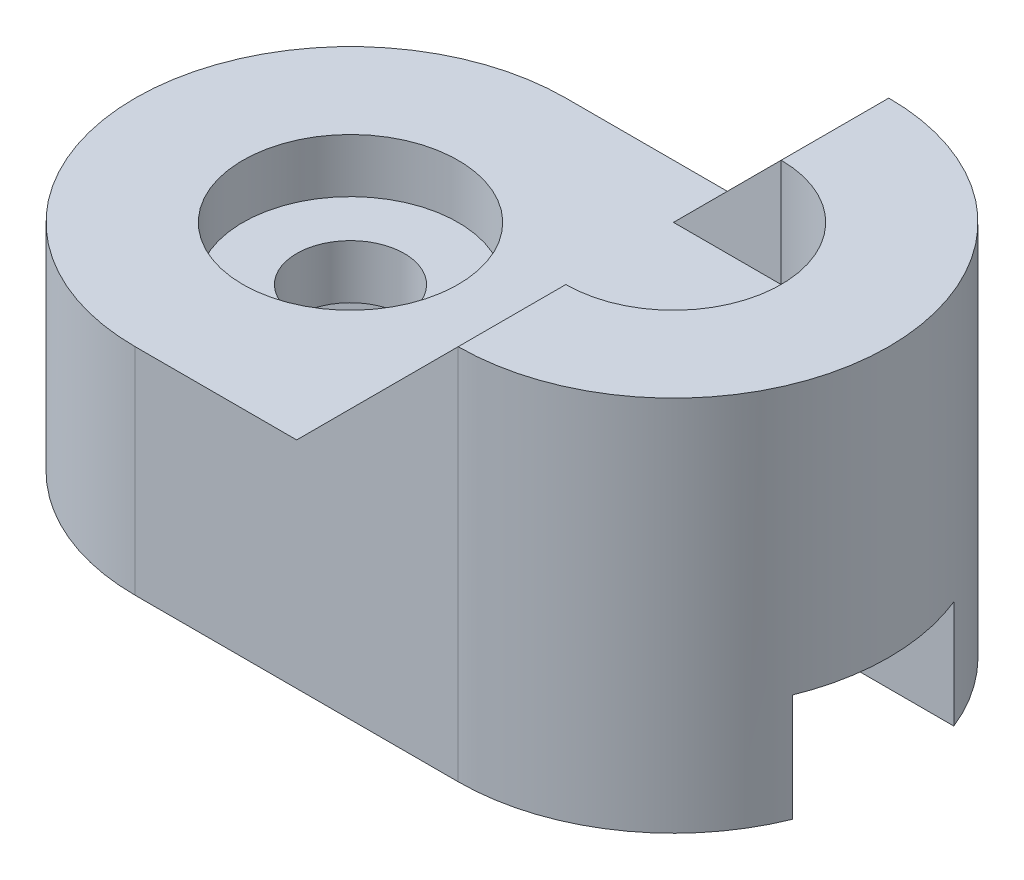
ISO-10303-21;
HEADER;
FILE_DESCRIPTION(('STEP AP214'),'2;1');
FILE_NAME('part.step','',(''),(''),'','','');
FILE_SCHEMA(('AUTOMOTIVE_DESIGN { 1 0 10303 214 1 1 1 1 }'));
ENDSEC;
DATA;
#1=APPLICATION_CONTEXT('core data for automotive mechanical design processes');
#2=APPLICATION_PROTOCOL_DEFINITION('international standard','automotive_design',2000,#1);
#3=PRODUCT_CONTEXT('',#1,'mechanical');
#4=PRODUCT('Part','Part','',(#3));
#5=PRODUCT_RELATED_PRODUCT_CATEGORY('part','',(#4));
#6=PRODUCT_DEFINITION_FORMATION('','',#4);
#7=PRODUCT_DEFINITION_CONTEXT('part definition',#1,'design');
#8=PRODUCT_DEFINITION('design','',#6,#7);
#9=PRODUCT_DEFINITION_SHAPE('','',#8);
#10=(LENGTH_UNIT() NAMED_UNIT(*) SI_UNIT(.MILLI.,.METRE.));
#11=(NAMED_UNIT(*) PLANE_ANGLE_UNIT() SI_UNIT($,.RADIAN.));
#12=(NAMED_UNIT(*) SI_UNIT($,.STERADIAN.) SOLID_ANGLE_UNIT());
#13=UNCERTAINTY_MEASURE_WITH_UNIT(LENGTH_MEASURE(1.E-05),#10,'distance_accuracy_value','');
#14=(GEOMETRIC_REPRESENTATION_CONTEXT(3) GLOBAL_UNCERTAINTY_ASSIGNED_CONTEXT((#13)) GLOBAL_UNIT_ASSIGNED_CONTEXT((#10,
#11,#12)) REPRESENTATION_CONTEXT('',''));
#15=CARTESIAN_POINT('',(0.,0.,0.));
#16=DIRECTION('',(0.,0.,1.));
#17=DIRECTION('',(1.,0.,0.));
#18=AXIS2_PLACEMENT_3D('',#15,#16,#17);
#19=CARTESIAN_POINT('',(0.,70.,-40.));
#20=DIRECTION('',(1.,0.,0.));
#21=DIRECTION('',(0.,0.,-1.));
#22=AXIS2_PLACEMENT_3D('',#19,#20,#21);
#23=PLANE('',#22);
#24=DIRECTION('',(0.,0.,1.));
#25=VECTOR('',#24,1.);
#26=CARTESIAN_POINT('',(0.,40.,-40.));
#27=LINE('',#26,#25);
#28=CARTESIAN_POINT('',(0.,40.,-30.));
#29=VERTEX_POINT('',#28);
#30=CARTESIAN_POINT('',(0.,40.,-20.));
#31=VERTEX_POINT('',#30);
#32=EDGE_CURVE('E167',#29,#31,#27,.T.);
#33=ORIENTED_EDGE('',*,*,#32,.T.);
#34=DIRECTION('',(0.,1.,0.));
#35=VECTOR('',#34,1.);
#36=CARTESIAN_POINT('',(0.,70.,-20.));
#37=LINE('',#36,#35);
#38=CARTESIAN_POINT('',(0.,70.,-20.));
#39=VERTEX_POINT('',#38);
#40=EDGE_CURVE('E52',#31,#39,#37,.T.);
#41=ORIENTED_EDGE('',*,*,#40,.T.);
#42=DIRECTION('',(0.,0.,1.));
#43=VECTOR('',#42,1.);
#44=CARTESIAN_POINT('',(0.,70.,-40.));
#45=LINE('',#44,#43);
#46=CARTESIAN_POINT('',(0.,70.,-30.));
#47=VERTEX_POINT('',#46);
#48=EDGE_CURVE('E154',#47,#39,#45,.T.);
#49=ORIENTED_EDGE('',*,*,#48,.F.);
#50=DIRECTION('',(0.,1.,0.));
#51=VECTOR('',#50,1.);
#52=CARTESIAN_POINT('',(0.,70.,-30.));
#53=LINE('',#52,#51);
#54=EDGE_CURVE('E236',#29,#47,#53,.T.);
#55=ORIENTED_EDGE('',*,*,#54,.F.);
#56=EDGE_LOOP('',(#33,#41,#49,#55));
#57=FACE_BOUND('',#56,.T.);
#58=ADVANCED_FACE('F39',(#57),#23,.F.);
#59=CARTESIAN_POINT('',(0.,70.,0.));
#60=DIRECTION('',(0.,-1.,0.));
#61=DIRECTION('',(0.,0.,-1.));
#62=AXIS2_PLACEMENT_3D('',#59,#60,#61);
#63=PLANE('',#62);
#64=CARTESIAN_POINT('',(0.,70.,0.));
#65=DIRECTION('',(0.,1.,0.));
#66=DIRECTION('',(0.,0.,1.));
#67=AXIS2_PLACEMENT_3D('',#64,#65,#66);
#68=CIRCLE('',#67,20.);
#69=CARTESIAN_POINT('',(0.,70.,20.));
#70=VERTEX_POINT('',#69);
#71=EDGE_CURVE('E143',#70,#39,#68,.T.);
#72=ORIENTED_EDGE('',*,*,#71,.F.);
#73=CARTESIAN_POINT('',(0.,70.,30.));
#74=VERTEX_POINT('',#73);
#75=EDGE_CURVE('E151',#70,#74,#45,.T.);
#76=ORIENTED_EDGE('',*,*,#75,.T.);
#77=DIRECTION('',(0.,0.,1.));
#78=VECTOR('',#77,1.);
#79=CARTESIAN_POINT('',(0.,70.,40.));
#80=LINE('',#79,#78);
#81=CARTESIAN_POINT('',(0.,70.,40.));
#82=VERTEX_POINT('',#81);
#83=EDGE_CURVE('E249',#74,#82,#80,.T.);
#84=ORIENTED_EDGE('',*,*,#83,.T.);
#85=CARTESIAN_POINT('',(0.,70.,0.));
#86=DIRECTION('',(0.,1.,0.));
#87=DIRECTION('',(0.,0.,-1.));
#88=AXIS2_PLACEMENT_3D('',#85,#86,#87);
#89=CIRCLE('',#88,40.);
#90=CARTESIAN_POINT('',(0.,70.,-40.));
#91=VERTEX_POINT('',#90);
#92=EDGE_CURVE('E165',#82,#91,#89,.T.);
#93=ORIENTED_EDGE('',*,*,#92,.T.);
#94=EDGE_CURVE('E163',#91,#47,#45,.T.);
#95=ORIENTED_EDGE('',*,*,#94,.T.);
#96=ORIENTED_EDGE('',*,*,#48,.T.);
#97=EDGE_LOOP('',(#72,#76,#84,#93,#95,#96));
#98=FACE_BOUND('',#97,.T.);
#99=ADVANCED_FACE('F149',(#98),#63,.F.);
#100=ORIENTED_EDGE('',*,*,#75,.F.);
#101=DIRECTION('',(0.,1.,0.));
#102=VECTOR('',#101,1.);
#103=CARTESIAN_POINT('',(0.,70.,20.));
#104=LINE('',#103,#102);
#105=CARTESIAN_POINT('',(0.,40.,20.));
#106=VERTEX_POINT('',#105);
#107=EDGE_CURVE('E140',#70,#106,#104,.F.);
#108=ORIENTED_EDGE('',*,*,#107,.T.);
#109=CARTESIAN_POINT('',(0.,40.,30.));
#110=VERTEX_POINT('',#109);
#111=EDGE_CURVE('E272',#106,#110,#27,.T.);
#112=ORIENTED_EDGE('',*,*,#111,.T.);
#113=DIRECTION('',(0.,-1.,0.));
#114=VECTOR('',#113,1.);
#115=CARTESIAN_POINT('',(0.,70.,30.));
#116=LINE('',#115,#114);
#117=EDGE_CURVE('E161',#74,#110,#116,.T.);
#118=ORIENTED_EDGE('',*,*,#117,.F.);
#119=EDGE_LOOP('',(#100,#108,#112,#118));
#120=FACE_BOUND('',#119,.T.);
#121=ADVANCED_FACE('F157',(#120),#23,.F.);
#122=CARTESIAN_POINT('',(0.,0.,0.));
#123=DIRECTION('',(0.,1.,0.));
#124=DIRECTION('',(0.,0.,1.));
#125=AXIS2_PLACEMENT_3D('',#122,#123,#124);
#126=PLANE('',#125);
#127=DIRECTION('',(1.,0.,0.));
#128=VECTOR('',#127,1.);
#129=CARTESIAN_POINT('',(0.,0.,40.));
#130=LINE('',#129,#128);
#131=CARTESIAN_POINT('',(-60.,0.,40.));
#132=VERTEX_POINT('',#131);
#133=CARTESIAN_POINT('',(0.,0.,40.));
#134=VERTEX_POINT('',#133);
#135=EDGE_CURVE('E187',#132,#134,#130,.T.);
#136=ORIENTED_EDGE('',*,*,#135,.F.);
#137=CARTESIAN_POINT('',(-60.,0.,0.));
#138=DIRECTION('',(0.,1.,0.));
#139=DIRECTION('',(0.,0.,1.));
#140=AXIS2_PLACEMENT_3D('',#137,#138,#139);
#141=CIRCLE('',#140,40.);
#142=CARTESIAN_POINT('',(-97.0809924354783,0.,15.));
#143=VERTEX_POINT('',#142);
#144=EDGE_CURVE('E181',#143,#132,#141,.T.);
#145=ORIENTED_EDGE('',*,*,#144,.F.);
#146=DIRECTION('',(1.,0.,0.));
#147=VECTOR('',#146,1.);
#148=CARTESIAN_POINT('',(0.,0.,15.));
#149=LINE('',#148,#147);
#150=CARTESIAN_POINT('',(37.0809924354783,0.,15.));
#151=VERTEX_POINT('',#150);
#152=EDGE_CURVE('E201',#143,#151,#149,.T.);
#153=ORIENTED_EDGE('',*,*,#152,.T.);
#154=CARTESIAN_POINT('',(0.,0.,0.));
#155=DIRECTION('',(0.,1.,0.));
#156=DIRECTION('',(0.,0.,1.));
#157=AXIS2_PLACEMENT_3D('',#154,#155,#156);
#158=CIRCLE('',#157,40.);
#159=EDGE_CURVE('E168',#134,#151,#158,.T.);
#160=ORIENTED_EDGE('',*,*,#159,.F.);
#161=EDGE_LOOP('',(#136,#145,#153,#160));
#162=FACE_BOUND('',#161,.T.);
#163=ADVANCED_FACE('F327',(#162),#126,.F.);
#164=CARTESIAN_POINT('',(0.,40.,0.));
#165=DIRECTION('',(0.,-1.,0.));
#166=DIRECTION('',(0.,0.,-1.));
#167=AXIS2_PLACEMENT_3D('',#164,#165,#166);
#168=CYLINDRICAL_SURFACE('',#167,40.);
#169=DIRECTION('',(0.,-1.,0.));
#170=VECTOR('',#169,1.);
#171=CARTESIAN_POINT('',(0.,40.,-40.));
#172=LINE('',#171,#170);
#173=CARTESIAN_POINT('',(0.,0.,-40.));
#174=VERTEX_POINT('',#173);
#175=EDGE_CURVE('E197',#91,#174,#172,.T.);
#176=ORIENTED_EDGE('',*,*,#175,.F.);
#177=ORIENTED_EDGE('',*,*,#92,.F.);
#178=DIRECTION('',(0.,-1.,0.));
#179=VECTOR('',#178,1.);
#180=CARTESIAN_POINT('',(0.,40.,40.));
#181=LINE('',#180,#179);
#182=EDGE_CURVE('E186',#82,#134,#181,.T.);
#183=ORIENTED_EDGE('',*,*,#182,.T.);
#184=ORIENTED_EDGE('',*,*,#159,.T.);
#185=DIRECTION('',(0.,-1.,0.));
#186=VECTOR('',#185,1.);
#187=CARTESIAN_POINT('',(37.0809924354783,40.,15.));
#188=LINE('',#187,#186);
#189=CARTESIAN_POINT('',(37.0809924354783,20.,15.));
#190=VERTEX_POINT('',#189);
#191=EDGE_CURVE('E267',#151,#190,#188,.F.);
#192=ORIENTED_EDGE('',*,*,#191,.T.);
#193=CARTESIAN_POINT('',(0.,20.,0.));
#194=DIRECTION('',(0.,1.,0.));
#195=DIRECTION('',(0.,0.,1.));
#196=AXIS2_PLACEMENT_3D('',#193,#194,#195);
#197=CIRCLE('',#196,40.);
#198=CARTESIAN_POINT('',(37.0809924354783,20.,-15.));
#199=VERTEX_POINT('',#198);
#200=EDGE_CURVE('E275',#190,#199,#197,.T.);
#201=ORIENTED_EDGE('',*,*,#200,.T.);
#202=DIRECTION('',(0.,-1.,0.));
#203=VECTOR('',#202,1.);
#204=CARTESIAN_POINT('',(37.0809924354783,40.,-15.));
#205=LINE('',#204,#203);
#206=CARTESIAN_POINT('',(37.0809924354783,0.,-15.));
#207=VERTEX_POINT('',#206);
#208=EDGE_CURVE('E262',#199,#207,#205,.T.);
#209=ORIENTED_EDGE('',*,*,#208,.T.);
#210=EDGE_CURVE('E166',#207,#174,#158,.T.);
#211=ORIENTED_EDGE('',*,*,#210,.T.);
#212=EDGE_LOOP('',(#176,#177,#183,#184,#192,#201,#209,#211));
#213=FACE_BOUND('',#212,.T.);
#214=ADVANCED_FACE('F41',(#213),#168,.T.);
#215=CARTESIAN_POINT('',(0.,40.,-40.));
#216=DIRECTION('',(0.,0.,1.));
#217=DIRECTION('',(1.,0.,0.));
#218=AXIS2_PLACEMENT_3D('',#215,#216,#217);
#219=PLANE('',#218);
#220=DIRECTION('',(-1.,0.,0.));
#221=VECTOR('',#220,1.);
#222=CARTESIAN_POINT('',(0.,0.,-40.));
#223=LINE('',#222,#221);
#224=CARTESIAN_POINT('',(-60.,0.,-40.));
#225=VERTEX_POINT('',#224);
#226=EDGE_CURVE('E179',#174,#225,#223,.T.);
#227=ORIENTED_EDGE('',*,*,#226,.T.);
#228=DIRECTION('',(0.,-1.,0.));
#229=VECTOR('',#228,1.);
#230=CARTESIAN_POINT('',(-60.,40.,-40.));
#231=LINE('',#230,#229);
#232=CARTESIAN_POINT('',(-60.,40.,-40.));
#233=VERTEX_POINT('',#232);
#234=EDGE_CURVE('E192',#233,#225,#231,.T.);
#235=ORIENTED_EDGE('',*,*,#234,.F.);
#236=DIRECTION('',(-1.,0.,0.));
#237=VECTOR('',#236,1.);
#238=CARTESIAN_POINT('',(0.,40.,-40.));
#239=LINE('',#238,#237);
#240=CARTESIAN_POINT('',(-30.,40.,-40.));
#241=VERTEX_POINT('',#240);
#242=EDGE_CURVE('E190',#241,#233,#239,.T.);
#243=ORIENTED_EDGE('',*,*,#242,.F.);
#244=DIRECTION('',(0.707106781186547,0.707106781186548,0.));
#245=VECTOR('',#244,1.);
#246=CARTESIAN_POINT('',(0.,70.,-40.));
#247=LINE('',#246,#245);
#248=EDGE_CURVE('E234',#241,#91,#247,.T.);
#249=ORIENTED_EDGE('',*,*,#248,.T.);
#250=ORIENTED_EDGE('',*,*,#175,.T.);
#251=EDGE_LOOP('',(#227,#235,#243,#249,#250));
#252=FACE_BOUND('',#251,.T.);
#253=ADVANCED_FACE('F299',(#252),#219,.F.);
#254=CARTESIAN_POINT('',(-60.,40.,0.));
#255=DIRECTION('',(0.,-1.,0.));
#256=DIRECTION('',(0.,0.,-1.));
#257=AXIS2_PLACEMENT_3D('',#254,#255,#256);
#258=CYLINDRICAL_SURFACE('',#257,40.);
#259=ORIENTED_EDGE('',*,*,#234,.T.);
#260=CARTESIAN_POINT('',(-97.0809924354783,0.,-15.));
#261=VERTEX_POINT('',#260);
#262=EDGE_CURVE('E184',#225,#261,#141,.T.);
#263=ORIENTED_EDGE('',*,*,#262,.T.);
#264=DIRECTION('',(0.,-1.,0.));
#265=VECTOR('',#264,1.);
#266=CARTESIAN_POINT('',(-97.0809924354783,40.,-15.));
#267=LINE('',#266,#265);
#268=CARTESIAN_POINT('',(-97.0809924354783,20.,-15.));
#269=VERTEX_POINT('',#268);
#270=EDGE_CURVE('E259',#261,#269,#267,.F.);
#271=ORIENTED_EDGE('',*,*,#270,.T.);
#272=CARTESIAN_POINT('',(-60.,20.,0.));
#273=DIRECTION('',(0.,1.,0.));
#274=DIRECTION('',(0.,0.,1.));
#275=AXIS2_PLACEMENT_3D('',#272,#273,#274);
#276=CIRCLE('',#275,40.);
#277=CARTESIAN_POINT('',(-97.0809924354783,20.,15.));
#278=VERTEX_POINT('',#277);
#279=EDGE_CURVE('E50',#269,#278,#276,.T.);
#280=ORIENTED_EDGE('',*,*,#279,.T.);
#281=DIRECTION('',(0.,-1.,0.));
#282=VECTOR('',#281,1.);
#283=CARTESIAN_POINT('',(-97.0809924354783,40.,15.));
#284=LINE('',#283,#282);
#285=EDGE_CURVE('E266',#278,#143,#284,.T.);
#286=ORIENTED_EDGE('',*,*,#285,.T.);
#287=ORIENTED_EDGE('',*,*,#144,.T.);
#288=DIRECTION('',(0.,-1.,0.));
#289=VECTOR('',#288,1.);
#290=CARTESIAN_POINT('',(-60.,40.,40.));
#291=LINE('',#290,#289);
#292=CARTESIAN_POINT('',(-60.,40.,40.));
#293=VERTEX_POINT('',#292);
#294=EDGE_CURVE('E191',#293,#132,#291,.T.);
#295=ORIENTED_EDGE('',*,*,#294,.F.);
#296=CARTESIAN_POINT('',(-60.,40.,0.));
#297=DIRECTION('',(0.,1.,0.));
#298=DIRECTION('',(0.,0.,1.));
#299=AXIS2_PLACEMENT_3D('',#296,#297,#298);
#300=CIRCLE('',#299,40.);
#301=EDGE_CURVE('E280',#233,#293,#300,.T.);
#302=ORIENTED_EDGE('',*,*,#301,.F.);
#303=EDGE_LOOP('',(#259,#263,#271,#280,#286,#287,#295,#302));
#304=FACE_BOUND('',#303,.T.);
#305=ADVANCED_FACE('F359',(#304),#258,.T.);
#306=CARTESIAN_POINT('',(0.,40.,40.));
#307=DIRECTION('',(0.,0.,-1.));
#308=DIRECTION('',(-1.,0.,0.));
#309=AXIS2_PLACEMENT_3D('',#306,#307,#308);
#310=PLANE('',#309);
#311=ORIENTED_EDGE('',*,*,#294,.T.);
#312=ORIENTED_EDGE('',*,*,#135,.T.);
#313=ORIENTED_EDGE('',*,*,#182,.F.);
#314=DIRECTION('',(0.707106781186547,0.707106781186548,0.));
#315=VECTOR('',#314,1.);
#316=CARTESIAN_POINT('',(0.,70.,40.));
#317=LINE('',#316,#315);
#318=CARTESIAN_POINT('',(-30.,40.,40.));
#319=VERTEX_POINT('',#318);
#320=EDGE_CURVE('E245',#319,#82,#317,.T.);
#321=ORIENTED_EDGE('',*,*,#320,.F.);
#322=DIRECTION('',(1.,0.,0.));
#323=VECTOR('',#322,1.);
#324=CARTESIAN_POINT('',(0.,40.,40.));
#325=LINE('',#324,#323);
#326=EDGE_CURVE('E178',#293,#319,#325,.T.);
#327=ORIENTED_EDGE('',*,*,#326,.F.);
#328=EDGE_LOOP('',(#311,#312,#313,#321,#327));
#329=FACE_BOUND('',#328,.T.);
#330=ADVANCED_FACE('F290',(#329),#310,.F.);
#331=CARTESIAN_POINT('',(0.,40.,0.));
#332=DIRECTION('',(0.,1.,0.));
#333=DIRECTION('',(0.,0.,1.));
#334=AXIS2_PLACEMENT_3D('',#331,#332,#333);
#335=PLANE('',#334);
#336=CARTESIAN_POINT('',(0.,40.,0.));
#337=DIRECTION('',(0.,1.,0.));
#338=DIRECTION('',(0.,0.,1.));
#339=AXIS2_PLACEMENT_3D('',#336,#337,#338);
#340=CIRCLE('',#339,20.);
#341=EDGE_CURVE('E11',#31,#106,#340,.T.);
#342=ORIENTED_EDGE('',*,*,#341,.F.);
#343=ORIENTED_EDGE('',*,*,#32,.F.);
#344=DIRECTION('',(-1.,0.,0.));
#345=VECTOR('',#344,1.);
#346=CARTESIAN_POINT('',(0.,40.,-30.));
#347=LINE('',#346,#345);
#348=CARTESIAN_POINT('',(-30.,40.,-30.));
#349=VERTEX_POINT('',#348);
#350=EDGE_CURVE('E233',#29,#349,#347,.T.);
#351=ORIENTED_EDGE('',*,*,#350,.T.);
#352=DIRECTION('',(0.,0.,1.));
#353=VECTOR('',#352,1.);
#354=CARTESIAN_POINT('',(-30.,40.,0.));
#355=LINE('',#354,#353);
#356=EDGE_CURVE('E238',#241,#349,#355,.T.);
#357=ORIENTED_EDGE('',*,*,#356,.F.);
#358=ORIENTED_EDGE('',*,*,#242,.T.);
#359=ORIENTED_EDGE('',*,*,#301,.T.);
#360=ORIENTED_EDGE('',*,*,#326,.T.);
#361=DIRECTION('',(0.,0.,-1.));
#362=VECTOR('',#361,1.);
#363=CARTESIAN_POINT('',(-30.,40.,0.));
#364=LINE('',#363,#362);
#365=CARTESIAN_POINT('',(-30.,40.,30.));
#366=VERTEX_POINT('',#365);
#367=EDGE_CURVE('E251',#366,#319,#364,.F.);
#368=ORIENTED_EDGE('',*,*,#367,.F.);
#369=DIRECTION('',(1.,0.,0.));
#370=VECTOR('',#369,1.);
#371=CARTESIAN_POINT('',(0.,40.,30.));
#372=LINE('',#371,#370);
#373=EDGE_CURVE('E247',#366,#110,#372,.T.);
#374=ORIENTED_EDGE('',*,*,#373,.T.);
#375=ORIENTED_EDGE('',*,*,#111,.F.);
#376=EDGE_LOOP('',(#342,#343,#351,#357,#358,#359,#360,#368,#374,#375));
#377=FACE_BOUND('',#376,.T.);
#378=CARTESIAN_POINT('',(-60.,40.,0.));
#379=DIRECTION('',(0.,1.,0.));
#380=DIRECTION('',(0.,0.,1.));
#381=AXIS2_PLACEMENT_3D('',#378,#379,#380);
#382=CIRCLE('',#381,20.);
#383=CARTESIAN_POINT('',(-60.,40.,20.));
#384=VERTEX_POINT('',#383);
#385=EDGE_CURVE('E224',#384,#384,#382,.T.);
#386=ORIENTED_EDGE('',*,*,#385,.F.);
#387=EDGE_LOOP('',(#386));
#388=FACE_BOUND('',#387,.T.);
#389=ADVANCED_FACE('F281',(#377,#388),#335,.T.);
#390=DIRECTION('',(-1.,0.,0.));
#391=VECTOR('',#390,1.);
#392=CARTESIAN_POINT('',(0.,0.,-15.));
#393=LINE('',#392,#391);
#394=EDGE_CURVE('E199',#207,#261,#393,.T.);
#395=ORIENTED_EDGE('',*,*,#394,.T.);
#396=ORIENTED_EDGE('',*,*,#262,.F.);
#397=ORIENTED_EDGE('',*,*,#226,.F.);
#398=ORIENTED_EDGE('',*,*,#210,.F.);
#399=EDGE_LOOP('',(#395,#396,#397,#398));
#400=FACE_BOUND('',#399,.T.);
#401=ADVANCED_FACE('F333',(#400),#126,.F.);
#402=CARTESIAN_POINT('',(-100.,20.,15.));
#403=DIRECTION('',(0.,1.,0.));
#404=DIRECTION('',(0.,0.,1.));
#405=AXIS2_PLACEMENT_3D('',#402,#403,#404);
#406=PLANE('',#405);
#407=CARTESIAN_POINT('',(0.,20.,0.));
#408=DIRECTION('',(0.,1.,0.));
#409=DIRECTION('',(0.,0.,1.));
#410=AXIS2_PLACEMENT_3D('',#407,#408,#409);
#411=CIRCLE('',#410,10.);
#412=CARTESIAN_POINT('',(0.,20.,10.));
#413=VERTEX_POINT('',#412);
#414=EDGE_CURVE('E144',#413,#413,#411,.T.);
#415=ORIENTED_EDGE('',*,*,#414,.T.);
#416=EDGE_LOOP('',(#415));
#417=FACE_BOUND('',#416,.T.);
#418=CARTESIAN_POINT('',(-60.,20.,0.));
#419=DIRECTION('',(0.,1.,0.));
#420=DIRECTION('',(0.,0.,1.));
#421=AXIS2_PLACEMENT_3D('',#418,#419,#420);
#422=CIRCLE('',#421,10.);
#423=CARTESIAN_POINT('',(-60.,20.,10.));
#424=VERTEX_POINT('',#423);
#425=EDGE_CURVE('E208',#424,#424,#422,.T.);
#426=ORIENTED_EDGE('',*,*,#425,.T.);
#427=EDGE_LOOP('',(#426));
#428=FACE_BOUND('',#427,.T.);
#429=DIRECTION('',(1.,0.,0.));
#430=VECTOR('',#429,1.);
#431=CARTESIAN_POINT('',(-100.,20.,15.));
#432=LINE('',#431,#430);
#433=EDGE_CURVE('E258',#278,#190,#432,.T.);
#434=ORIENTED_EDGE('',*,*,#433,.F.);
#435=ORIENTED_EDGE('',*,*,#279,.F.);
#436=DIRECTION('',(1.,0.,0.));
#437=VECTOR('',#436,1.);
#438=CARTESIAN_POINT('',(-100.,20.,-15.));
#439=LINE('',#438,#437);
#440=EDGE_CURVE('E254',#269,#199,#439,.T.);
#441=ORIENTED_EDGE('',*,*,#440,.T.);
#442=ORIENTED_EDGE('',*,*,#200,.F.);
#443=EDGE_LOOP('',(#434,#435,#441,#442));
#444=FACE_BOUND('',#443,.T.);
#445=ADVANCED_FACE('F345',(#417,#428,#444),#406,.F.);
#446=CARTESIAN_POINT('',(-100.,0.,15.));
#447=DIRECTION('',(0.,0.,1.));
#448=DIRECTION('',(1.,0.,0.));
#449=AXIS2_PLACEMENT_3D('',#446,#447,#448);
#450=PLANE('',#449);
#451=ORIENTED_EDGE('',*,*,#152,.F.);
#452=ORIENTED_EDGE('',*,*,#285,.F.);
#453=ORIENTED_EDGE('',*,*,#433,.T.);
#454=ORIENTED_EDGE('',*,*,#191,.F.);
#455=EDGE_LOOP('',(#451,#452,#453,#454));
#456=FACE_BOUND('',#455,.T.);
#457=ADVANCED_FACE('F349',(#456),#450,.F.);
#458=CARTESIAN_POINT('',(-100.,0.,-15.));
#459=DIRECTION('',(0.,0.,-1.));
#460=DIRECTION('',(-1.,0.,0.));
#461=AXIS2_PLACEMENT_3D('',#458,#459,#460);
#462=PLANE('',#461);
#463=ORIENTED_EDGE('',*,*,#440,.F.);
#464=ORIENTED_EDGE('',*,*,#270,.F.);
#465=ORIENTED_EDGE('',*,*,#394,.F.);
#466=ORIENTED_EDGE('',*,*,#208,.F.);
#467=EDGE_LOOP('',(#463,#464,#465,#466));
#468=FACE_BOUND('',#467,.T.);
#469=ADVANCED_FACE('F351',(#468),#462,.F.);
#470=CARTESIAN_POINT('',(0.,70.,40.));
#471=DIRECTION('',(0.707106781186548,-0.707106781186547,0.));
#472=DIRECTION('',(0.707106781186547,0.707106781186548,0.));
#473=AXIS2_PLACEMENT_3D('',#470,#471,#472);
#474=PLANE('',#473);
#475=DIRECTION('',(0.707106781186547,0.707106781186548,0.));
#476=VECTOR('',#475,1.);
#477=CARTESIAN_POINT('',(0.,70.,30.));
#478=LINE('',#477,#476);
#479=EDGE_CURVE('E244',#366,#74,#478,.T.);
#480=ORIENTED_EDGE('',*,*,#479,.F.);
#481=ORIENTED_EDGE('',*,*,#367,.T.);
#482=ORIENTED_EDGE('',*,*,#320,.T.);
#483=ORIENTED_EDGE('',*,*,#83,.F.);
#484=EDGE_LOOP('',(#480,#481,#482,#483));
#485=FACE_BOUND('',#484,.T.);
#486=ADVANCED_FACE('F291',(#485),#474,.F.);
#487=CARTESIAN_POINT('',(-30.,35.,30.));
#488=DIRECTION('',(0.,0.,1.));
#489=DIRECTION('',(1.,0.,0.));
#490=AXIS2_PLACEMENT_3D('',#487,#488,#489);
#491=PLANE('',#490);
#492=ORIENTED_EDGE('',*,*,#373,.F.);
#493=ORIENTED_EDGE('',*,*,#479,.T.);
#494=ORIENTED_EDGE('',*,*,#117,.T.);
#495=EDGE_LOOP('',(#492,#493,#494));
#496=FACE_BOUND('',#495,.T.);
#497=ADVANCED_FACE('F314',(#496),#491,.F.);
#498=CARTESIAN_POINT('',(-30.,35.,-30.));
#499=DIRECTION('',(0.,0.,-1.));
#500=DIRECTION('',(-1.,0.,0.));
#501=AXIS2_PLACEMENT_3D('',#498,#499,#500);
#502=PLANE('',#501);
#503=ORIENTED_EDGE('',*,*,#350,.F.);
#504=ORIENTED_EDGE('',*,*,#54,.T.);
#505=DIRECTION('',(0.707106781186547,0.707106781186548,0.));
#506=VECTOR('',#505,1.);
#507=CARTESIAN_POINT('',(0.,70.,-30.));
#508=LINE('',#507,#506);
#509=EDGE_CURVE('E62',#349,#47,#508,.T.);
#510=ORIENTED_EDGE('',*,*,#509,.F.);
#511=EDGE_LOOP('',(#503,#504,#510));
#512=FACE_BOUND('',#511,.T.);
#513=ADVANCED_FACE('F302',(#512),#502,.F.);
#514=CARTESIAN_POINT('',(0.,70.,-40.));
#515=DIRECTION('',(-0.707106781186548,0.707106781186547,0.));
#516=DIRECTION('',(0.707106781186547,0.707106781186548,0.));
#517=AXIS2_PLACEMENT_3D('',#514,#515,#516);
#518=PLANE('',#517);
#519=ORIENTED_EDGE('',*,*,#248,.F.);
#520=ORIENTED_EDGE('',*,*,#356,.T.);
#521=ORIENTED_EDGE('',*,*,#509,.T.);
#522=ORIENTED_EDGE('',*,*,#94,.F.);
#523=EDGE_LOOP('',(#519,#520,#521,#522));
#524=FACE_BOUND('',#523,.T.);
#525=ADVANCED_FACE('F301',(#524),#518,.T.);
#526=CARTESIAN_POINT('',(-60.,40.,0.));
#527=DIRECTION('',(0.,1.,0.));
#528=DIRECTION('',(0.,0.,1.));
#529=AXIS2_PLACEMENT_3D('',#526,#527,#528);
#530=CYLINDRICAL_SURFACE('',#529,10.);
#531=CARTESIAN_POINT('',(-60.,30.,0.));
#532=DIRECTION('',(0.,1.,0.));
#533=DIRECTION('',(0.,0.,1.));
#534=AXIS2_PLACEMENT_3D('',#531,#532,#533);
#535=CIRCLE('',#534,10.);
#536=CARTESIAN_POINT('',(-60.,30.,10.));
#537=VERTEX_POINT('',#536);
#538=EDGE_CURVE('E209',#537,#537,#535,.T.);
#539=ORIENTED_EDGE('',*,*,#538,.T.);
#540=EDGE_LOOP('',(#539));
#541=FACE_BOUND('',#540,.T.);
#542=ORIENTED_EDGE('',*,*,#425,.F.);
#543=EDGE_LOOP('',(#542));
#544=FACE_BOUND('',#543,.T.);
#545=ADVANCED_FACE('F303',(#541,#544),#530,.F.);
#546=CARTESIAN_POINT('',(-50.,30.,0.));
#547=DIRECTION('',(0.,-1.,0.));
#548=DIRECTION('',(0.,0.,-1.));
#549=AXIS2_PLACEMENT_3D('',#546,#547,#548);
#550=PLANE('',#549);
#551=ORIENTED_EDGE('',*,*,#538,.F.);
#552=EDGE_LOOP('',(#551));
#553=FACE_BOUND('',#552,.T.);
#554=CARTESIAN_POINT('',(-60.,30.,0.));
#555=DIRECTION('',(0.,1.,0.));
#556=DIRECTION('',(0.,0.,1.));
#557=AXIS2_PLACEMENT_3D('',#554,#555,#556);
#558=CIRCLE('',#557,20.);
#559=CARTESIAN_POINT('',(-60.,30.,20.));
#560=VERTEX_POINT('',#559);
#561=EDGE_CURVE('E227',#560,#560,#558,.T.);
#562=ORIENTED_EDGE('',*,*,#561,.T.);
#563=EDGE_LOOP('',(#562));
#564=FACE_BOUND('',#563,.T.);
#565=ADVANCED_FACE('F313',(#553,#564),#550,.F.);
#566=CARTESIAN_POINT('',(-60.,40.,0.));
#567=DIRECTION('',(0.,1.,0.));
#568=DIRECTION('',(0.,0.,1.));
#569=AXIS2_PLACEMENT_3D('',#566,#567,#568);
#570=CYLINDRICAL_SURFACE('',#569,20.);
#571=ORIENTED_EDGE('',*,*,#561,.F.);
#572=EDGE_LOOP('',(#571));
#573=FACE_BOUND('',#572,.T.);
#574=ORIENTED_EDGE('',*,*,#385,.T.);
#575=EDGE_LOOP('',(#574));
#576=FACE_BOUND('',#575,.T.);
#577=ADVANCED_FACE('F463',(#573,#576),#570,.F.);
#578=CARTESIAN_POINT('',(0.,70.,0.));
#579=DIRECTION('',(0.,1.,0.));
#580=DIRECTION('',(0.,0.,1.));
#581=AXIS2_PLACEMENT_3D('',#578,#579,#580);
#582=CYLINDRICAL_SURFACE('',#581,20.);
#583=CARTESIAN_POINT('',(0.,30.,0.));
#584=DIRECTION('',(0.,1.,0.));
#585=DIRECTION('',(0.,0.,1.));
#586=AXIS2_PLACEMENT_3D('',#583,#584,#585);
#587=CIRCLE('',#586,20.);
#588=CARTESIAN_POINT('',(0.,30.,20.));
#589=VERTEX_POINT('',#588);
#590=EDGE_CURVE('E156',#589,#589,#587,.T.);
#591=ORIENTED_EDGE('',*,*,#590,.F.);
#592=EDGE_LOOP('',(#591));
#593=FACE_BOUND('',#592,.T.);
#594=ORIENTED_EDGE('',*,*,#341,.T.);
#595=ORIENTED_EDGE('',*,*,#107,.F.);
#596=ORIENTED_EDGE('',*,*,#71,.T.);
#597=ORIENTED_EDGE('',*,*,#40,.F.);
#598=EDGE_LOOP('',(#594,#595,#596,#597));
#599=FACE_BOUND('',#598,.T.);
#600=ADVANCED_FACE('F137',(#593,#599),#582,.F.);
#601=CARTESIAN_POINT('',(0.,70.,0.));
#602=DIRECTION('',(0.,1.,0.));
#603=DIRECTION('',(0.,0.,1.));
#604=AXIS2_PLACEMENT_3D('',#601,#602,#603);
#605=CYLINDRICAL_SURFACE('',#604,10.);
#606=CARTESIAN_POINT('',(0.,30.,0.));
#607=DIRECTION('',(0.,1.,0.));
#608=DIRECTION('',(0.,0.,1.));
#609=AXIS2_PLACEMENT_3D('',#606,#607,#608);
#610=CIRCLE('',#609,10.);
#611=CARTESIAN_POINT('',(0.,30.,10.));
#612=VERTEX_POINT('',#611);
#613=EDGE_CURVE('E215',#612,#612,#610,.T.);
#614=ORIENTED_EDGE('',*,*,#613,.T.);
#615=EDGE_LOOP('',(#614));
#616=FACE_BOUND('',#615,.T.);
#617=ORIENTED_EDGE('',*,*,#414,.F.);
#618=EDGE_LOOP('',(#617));
#619=FACE_BOUND('',#618,.T.);
#620=ADVANCED_FACE('F491',(#616,#619),#605,.F.);
#621=CARTESIAN_POINT('',(10.,30.,0.));
#622=DIRECTION('',(0.,-1.,0.));
#623=DIRECTION('',(0.,0.,-1.));
#624=AXIS2_PLACEMENT_3D('',#621,#622,#623);
#625=PLANE('',#624);
#626=ORIENTED_EDGE('',*,*,#613,.F.);
#627=EDGE_LOOP('',(#626));
#628=FACE_BOUND('',#627,.T.);
#629=ORIENTED_EDGE('',*,*,#590,.T.);
#630=EDGE_LOOP('',(#629));
#631=FACE_BOUND('',#630,.T.);
#632=ADVANCED_FACE('F498',(#628,#631),#625,.F.);
#633=CLOSED_SHELL('',(#58,#99,#121,#163,#214,#253,#305,#330,#389,#401,#445,#457,#469,#486,#497,
#513,#525,#545,#565,#577,#600,#620,#632));
#634=MANIFOLD_SOLID_BREP('B2',#633);
#635=ADVANCED_BREP_SHAPE_REPRESENTATION('',(#18,#634),#14);
#636=SHAPE_DEFINITION_REPRESENTATION(#9,#635);
ENDSEC;
END-ISO-10303-21;
